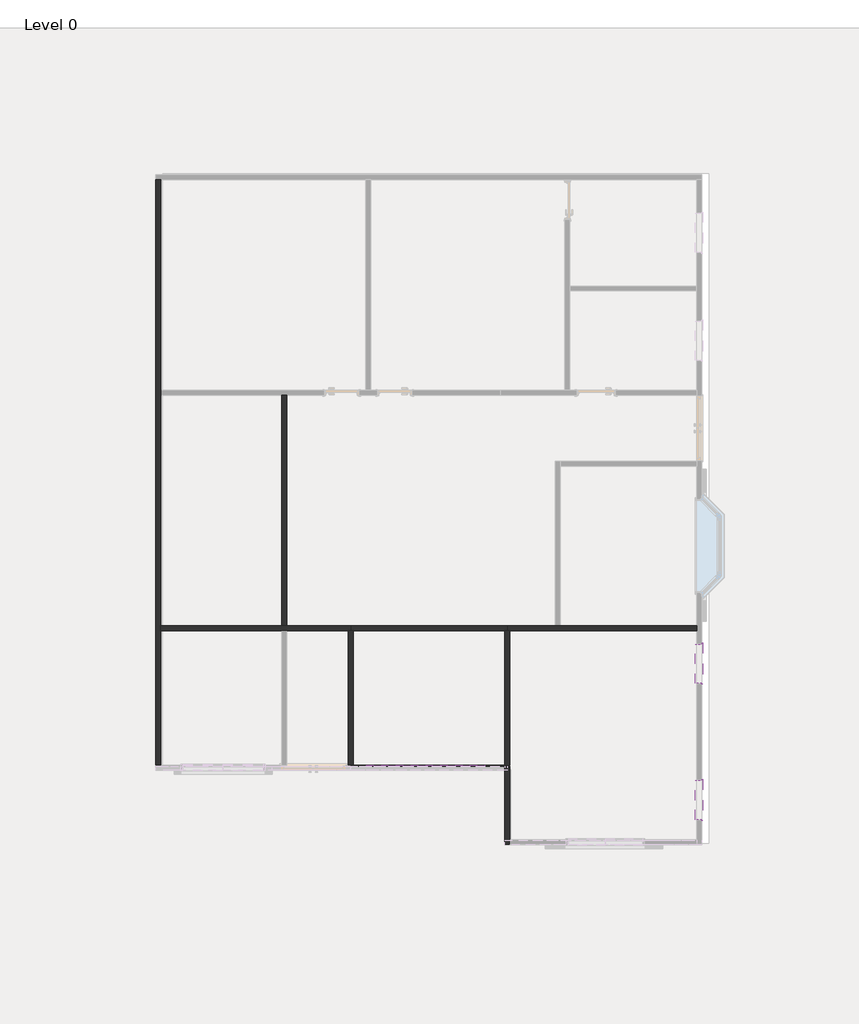
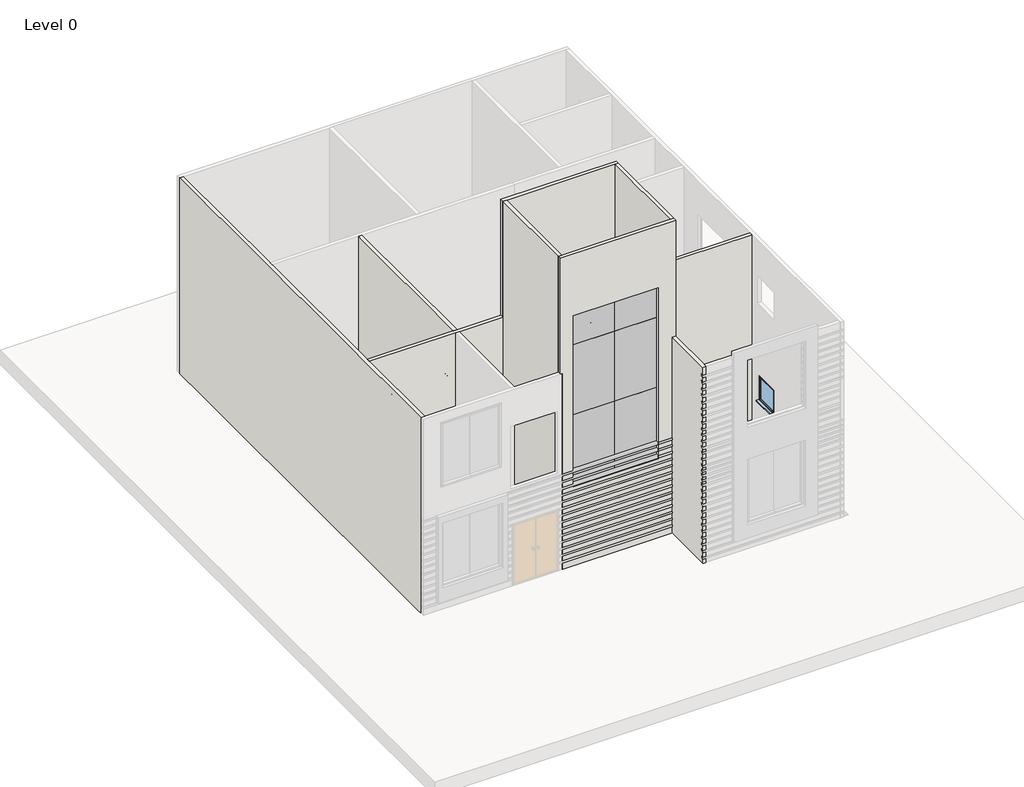
# One storey, part 3 of 5: 10 walls, 6 plates, 2 windows.
"""IFC4 building model written with IfcOpenShell, lengths in millimetres."""

from ifc_helpers import new_model, si_unit, origin, origin_with_axes, place, context, project, spatial, polyline, outline, extrude, faceted_brep, transform, mapped, element, save
from components import system_panel_glazed_fc6345c6, system_panel_glazed_e2854511, windows_sgl_plain_910x910mm_53772929

model = new_model("IFC4")

# Units and contexts
model_context = context("Model", 3, world=origin())
ifc_project = project(units=[si_unit("LENGTHUNIT", "METRE", prefix="MILLI")], contexts=[model_context])

# Site, building, storey
site = spatial("IfcSite", under=ifc_project)
building = spatial("IfcBuilding", under=site)
storey = spatial("IfcBuildingStorey", under=building, Name="Level 0", Elevation=0.0)

# Plates
placement = place(None, origin())
system_panel_glazed_shape = system_panel_glazed_fc6345c6(model_context)
element("IfcPlate", 1, ObjectType="System Panel : Glazed", at=placement, inside=storey, context=model_context, shape_type="MappedRepresentation", body=[
    mapped(system_panel_glazed_shape, transform((-13862.829089, -2815.8968048, 2700.0), x_axis=(1.0, 0.0, 0.0), y_axis=(0.0, 1.0, 0.0), z_axis=(0.0, 0.0, 1.0))),
])
element("IfcPlate", 2, ObjectType="System Panel : Glazed", at=placement, inside=storey, context=model_context, shape_type="MappedRepresentation", body=[
    mapped(system_panel_glazed_shape, transform((-12491.229089, -2815.8968048, 2700.0), x_axis=(1.0, 0.0, 0.0), y_axis=(0.0, 1.0, 0.0), z_axis=(0.0, 0.0, 1.0))),
])
element("IfcPlate", 3, ObjectType="System Panel : Glazed", at=placement, inside=storey, context=model_context, shape_type="MappedRepresentation", body=[
    mapped(system_panel_glazed_shape, transform((-13862.829089, -2815.8968048, 5100.0), x_axis=(1.0, 0.0, 0.0), y_axis=(0.0, 1.0, 0.0), z_axis=(0.0, 0.0, 1.0))),
])
element("IfcPlate", 4, ObjectType="System Panel : Glazed", at=placement, inside=storey, context=model_context, shape_type="MappedRepresentation", body=[
    mapped(system_panel_glazed_shape, transform((-12491.229089, -2815.8968048, 5100.0), x_axis=(1.0, 0.0, 0.0), y_axis=(0.0, 1.0, 0.0), z_axis=(0.0, 0.0, 1.0))),
])
system_panel_glazed_2_shape = system_panel_glazed_e2854511(model_context)
element("IfcPlate", 5, ObjectType="System Panel : Glazed", at=placement, inside=storey, context=model_context, shape_type="MappedRepresentation", body=[
    mapped(system_panel_glazed_2_shape, transform((-13862.829089, -2815.8968048, 7500.0), x_axis=(1.0, 0.0, 0.0), y_axis=(0.0, 1.0, 0.0), z_axis=(0.0, 0.0, 1.0))),
])
element("IfcPlate", 6, ObjectType="System Panel : Glazed", at=placement, inside=storey, context=model_context, shape_type="MappedRepresentation", body=[
    mapped(system_panel_glazed_2_shape, transform((-12491.229089, -2815.8968048, 7500.0), x_axis=(1.0, 0.0, 0.0), y_axis=(0.0, 1.0, 0.0), z_axis=(0.0, 0.0, 1.0))),
])

# Walls
element("IfcWall", 7, ObjectType="basic wall", at=placement, inside=storey, context=model_context, shape_type="Brep", body=[
    faceted_brep([(-19412.729089, 10785.8031952, 0.0), (-19412.729089, -2758.7468048, 0.0), (-19412.729089, -2758.7468048, 6705.6), (-19412.729089, 10785.8031952, 6705.6), (-19298.429089, 10785.8031952, 0.0), (-19298.429089, 10785.8031952, 6705.6), (-19298.429089, 5909.0031952, 6705.6), (-19298.429089, 5794.7031952, 6705.6), (-19298.429089, 460.7031952, 6705.6), (-19298.429089, 346.4031952, 6705.6), (-19298.429089, -2758.7468048, 6705.6), (-19298.429089, -2758.7468048, 0.0), (-19298.429089, 346.4031952, 0.0), (-19298.429089, 460.7031952, 0.0), (-19298.429089, 5794.7031952, 0.0), (-19298.429089, 5909.0031952, 0.0)], [[[0, 1, 2, 3]], [[4, 5, 6, 7, 8, 9, 10, 11, 12, 13, 14, 15]], [[1, 0, 4, 15, 14, 13, 12, 11]], [[3, 2, 10, 9, 8, 7, 6, 5]], [[0, 3, 5, 4]], [[1, 11, 10, 2]]]),
])
element("IfcWall", 8, ObjectType="basic wall", at=placement, inside=storey, context=model_context, shape_type="Brep", body=[
    faceted_brep([(-11348.229089, 346.4031952, 10668.0), (-11348.229089, 346.4031952, 0.0), (-11348.229089, -2758.7468048, 0.0), (-11348.229089, -2758.7468048, 10668.0), (-11233.929089, 346.4031952, 0.0), (-11233.929089, 346.4031952, 6705.6), (-11233.929089, 346.4031952, 10668.0), (-11233.929089, -2758.7468048, 10668.0), (-11233.929089, -2758.7468048, 6705.6), (-11233.929089, -2758.7468048, 0.0), (-11291.079089, 346.4031952, 0.0)], [[[0, 1, 2, 3]], [[4, 5, 6, 7, 8, 9]], [[2, 1, 10, 4, 9]], [[0, 3, 7, 6]], [[0, 6, 5, 4, 10, 1]], [[3, 2, 9, 8, 7]]]),
])
element("IfcWall", 9, ObjectType="basic wall", at=placement, inside=storey, context=model_context, shape_type="Brep", body=[
    faceted_brep([(-6903.229089, 460.7031952, 0.0), (-10065.529089, 460.7031952, 0.0), (-10179.829089, 460.7031952, 0.0), (-11291.079089, 460.7031952, 0.0), (-11291.079089, 460.7031952, 6705.6), (-11233.929089, 460.7031952, 6705.6), (-10179.829089, 460.7031952, 6705.6), (-10065.529089, 460.7031952, 6705.6), (-6903.229089, 460.7031952, 6705.6), (-6903.229089, 346.4031952, 0.0), (-6903.229089, 346.4031952, 6705.6), (-11233.929089, 346.4031952, 6705.6), (-11291.079089, 346.4031952, 6705.6), (-11291.079089, 346.4031952, 0.0), (-11233.929089, 346.4031952, 0.0)], [[[0, 1, 2, 3, 4, 5, 6, 7, 8]], [[9, 10, 11, 12, 13, 14]], [[3, 2, 1, 0, 9, 14, 13]], [[4, 3, 13, 12]], [[8, 7, 6, 5, 4, 12, 11, 10]], [[0, 8, 10, 9]]]),
])
element("IfcWall", 10, ObjectType="basic wall", at=placement, inside=storey, context=model_context, shape_type="Brep", body=[
    faceted_brep([(-14967.729089, 346.4031952, 10668.0), (-14967.729089, 346.4031952, 6705.6), (-14967.729089, 346.4031952, 0.0), (-14967.729089, -2758.7468048, 0.0), (-14967.729089, -2758.7468048, 6705.6), (-14967.729089, -2758.7468048, 10668.0), (-14853.429089, 346.4031952, 0.0), (-14853.429089, 346.4031952, 10668.0), (-14853.429089, -2758.7468048, 10668.0), (-14853.429089, -2758.7468048, 0.0), (-14910.579089, 346.4031952, 0.0), (-14910.579089, -2758.7468048, 0.0)], [[[0, 1, 2, 3, 4, 5]], [[6, 7, 8, 9]], [[3, 2, 10, 6, 9, 11]], [[0, 5, 8, 7]], [[0, 7, 6, 10, 2, 1]], [[3, 11, 9, 8, 5, 4]]]),
])
element("IfcWall", 11, ObjectType="basic wall", at=placement, inside=storey, context=model_context, shape_type="SweptSolid", body=[
    extrude(outline(polyline([(-16504.429089, 460.7031952), (-16504.429089, 5794.7031952), (-16390.129089, 5794.7031952), (-16390.129089, 460.7031952), (-16504.429089, 460.7031952)])), origin_with_axes(), (0.0, 0.0, 1.0), 6705.6),
])
element("IfcWall", 12, ObjectType="basic wall", at=placement, inside=storey, context=model_context, shape_type="Brep", body=[
    faceted_brep([(-14910.579089, 460.7031952, 0.0), (-16390.129089, 460.7031952, 0.0), (-16504.429089, 460.7031952, 0.0), (-19298.429089, 460.7031952, 0.0), (-19298.429089, 460.7031952, 6705.6), (-16504.429089, 460.7031952, 6705.6), (-16390.129089, 460.7031952, 6705.6), (-14967.729089, 460.7031952, 6705.6), (-14910.579089, 460.7031952, 6705.6), (-14910.579089, 346.4031952, 0.0), (-14910.579089, 346.4031952, 6705.6), (-14967.729089, 346.4031952, 6705.6), (-16390.129089, 346.4031952, 6705.6), (-16504.429089, 346.4031952, 6705.6), (-19298.429089, 346.4031952, 6705.6), (-19298.429089, 346.4031952, 0.0), (-16504.429089, 346.4031952, 0.0), (-16390.129089, 346.4031952, 0.0), (-14967.729089, 346.4031952, 0.0)], [[[0, 1, 2, 3, 4, 5, 6, 7, 8]], [[9, 10, 11, 12, 13, 14, 15, 16, 17, 18]], [[3, 2, 1, 0, 9, 18, 17, 16, 15]], [[8, 7, 6, 5, 4, 14, 13, 12, 11, 10]], [[0, 8, 10, 9]], [[4, 3, 15, 14]]]),
])
element("IfcWall", 13, ObjectType="basic wall", at=placement, inside=storey, context=model_context, shape_type="Brep", body=[
    faceted_brep([(-11291.079089, 460.7031952, 0.0), (-14910.579089, 460.7031952, 0.0), (-14910.579089, 460.7031952, 6705.6), (-14967.729089, 460.7031952, 6705.6), (-14967.729089, 460.7031952, 10668.0), (-11233.929089, 460.7031952, 10668.0), (-11233.929089, 460.7031952, 6705.6), (-11291.079089, 460.7031952, 6705.6), (-11291.079089, 346.4031952, 0.0), (-11291.079089, 346.4031952, 6705.6), (-11233.929089, 346.4031952, 6705.6), (-11233.929089, 346.4031952, 10668.0), (-11348.229089, 346.4031952, 10668.0), (-14853.429089, 346.4031952, 10668.0), (-14967.729089, 346.4031952, 10668.0), (-14967.729089, 346.4031952, 6705.6), (-14910.579089, 346.4031952, 6705.6), (-14910.579089, 346.4031952, 0.0), (-14853.429089, 346.4031952, 0.0), (-11348.229089, 346.4031952, 0.0)], [[[0, 1, 2, 3, 4, 5, 6, 7]], [[8, 9, 10, 11, 12, 13, 14, 15, 16, 17, 18, 19]], [[1, 0, 8, 19, 18, 17]], [[5, 4, 14, 13, 12, 11]], [[0, 7, 9, 8]], [[6, 10, 9, 7]], [[6, 5, 11, 10]], [[2, 1, 17, 16]], [[15, 3, 2, 16]], [[4, 3, 15, 14]]]),
])
element("IfcWall", 14, ObjectType="basic wall", at=placement, inside=storey, context=model_context, shape_type="Brep", body=[
    faceted_brep([(-11348.229089, -2815.8968048, 0.0), (-11348.229089, -2873.0468048, 0.0), (-11348.229089, -4593.8968048, 0.0), (-11348.229089, -4593.8968048, 152.4), (-11348.229089, -4501.3968048, 152.4), (-11348.229089, -4501.3968048, 227.4), (-11348.229089, -4583.8968048, 227.4), (-11348.229089, -4593.8968048, 217.4), (-11348.229089, -4593.8968048, 381.0), (-11348.229089, -4501.3968048, 381.0), (-11348.229089, -4501.3968048, 456.0), (-11348.229089, -4583.8968048, 456.0), (-11348.229089, -4593.8968048, 446.0), (-11348.229089, -4593.8968048, 609.6), (-11348.229089, -4501.3968048, 609.6), (-11348.229089, -4501.3968048, 684.6), (-11348.229089, -4583.8968048, 684.6), (-11348.229089, -4593.8968048, 674.6), (-11348.229089, -4593.8968048, 830.4106439), (-11348.229089, -4501.3968048, 830.4106439), (-11348.229089, -4501.3968048, 905.4106439), (-11348.229089, -4583.8968048, 905.4106439), (-11348.229089, -4593.8968048, 895.4106439), (-11348.229089, -4593.8968048, 1059.0106439), (-11348.229089, -4501.3968048, 1059.0106439), (-11348.229089, -4501.3968048, 1134.0106439), (-11348.229089, -4583.8968048, 1134.0106439), (-11348.229089, -4593.8968048, 1124.0106439), (-11348.229089, -4593.8968048, 1279.8212878), (-11348.229089, -4501.3968048, 1279.8212878), (-11348.229089, -4501.3968048, 1354.8212878), (-11348.229089, -4583.8968048, 1354.8212878), (-11348.229089, -4593.8968048, 1344.8212878), (-11348.229089, -4593.8968048, 1500.6319317), (-11348.229089, -4501.3968048, 1500.6319317), (-11348.229089, -4501.3968048, 1575.6319317), (-11348.229089, -4583.8968048, 1575.6319317), (-11348.229089, -4593.8968048, 1565.6319317), (-11348.229089, -4593.8968048, 1729.2319317), (-11348.229089, -4501.3968048, 1729.2319317), (-11348.229089, -4501.3968048, 1804.2319317), (-11348.229089, -4583.8968048, 1804.2319317), (-11348.229089, -4593.8968048, 1794.2319317), (-11348.229089, -4593.8968048, 1957.8319317), (-11348.229089, -4501.3968048, 1957.8319317), (-11348.229089, -4501.3968048, 2032.8319317), (-11348.229089, -4583.8968048, 2032.8319317), (-11348.229089, -4593.8968048, 2022.8319317), (-11348.229089, -4593.8968048, 2186.4319317), (-11348.229089, -4501.3968048, 2186.4319317), (-11348.229089, -4501.3968048, 2261.4319317), (-11348.229089, -4583.8968048, 2261.4319317), (-11348.229089, -4593.8968048, 2251.4319317), (-11348.229089, -4593.8968048, 2415.0319317), (-11348.229089, -4501.3968048, 2415.0319317), (-11348.229089, -4501.3968048, 2490.0319317), (-11348.229089, -4583.8968048, 2490.0319317), (-11348.229089, -4593.8968048, 2480.0319317), (-11348.229089, -4593.8968048, 2643.6319317), (-11348.229089, -4501.3968048, 2643.6319317), (-11348.229089, -4501.3968048, 2718.6319317), (-11348.229089, -4583.8968048, 2718.6319317), (-11348.229089, -4593.8968048, 2708.6319317), (-11348.229089, -4593.8968048, 2805.2765418), (-11348.229089, -4501.3968048, 2805.2765418), (-11348.229089, -4501.3968048, 2880.2765418), (-11348.229089, -4583.8968048, 2880.2765418), (-11348.229089, -4593.8968048, 2870.2765418), (-11348.229089, -4593.8968048, 2966.921152), (-11348.229089, -4501.3968048, 2966.921152), (-11348.229089, -4501.3968048, 3041.921152), (-11348.229089, -4583.8968048, 3041.921152), (-11348.229089, -4593.8968048, 3031.921152), (-11348.229089, -4593.8968048, 3128.5657622), (-11348.229089, -4501.3968048, 3128.5657622), (-11348.229089, -4501.3968048, 3203.5657622), (-11348.229089, -4583.8968048, 3203.5657622), (-11348.229089, -4593.8968048, 3193.5657622), (-11348.229089, -4593.8968048, 3290.2103724), (-11348.229089, -4501.3968048, 3290.2103724), (-11348.229089, -4501.3968048, 3365.2103724), (-11348.229089, -4583.8968048, 3365.2103724), (-11348.229089, -4593.8968048, 3355.2103724), (-11348.229089, -4593.8968048, 3518.8103724), (-11348.229089, -4501.3968048, 3518.8103724), (-11348.229089, -4501.3968048, 3593.8103724), (-11348.229089, -4583.8968048, 3593.8103724), (-11348.229089, -4593.8968048, 3583.8103724), (-11348.229089, -4593.8968048, 3747.4103724), (-11348.229089, -4501.3968048, 3747.4103724), (-11348.229089, -4501.3968048, 3822.4103724), (-11348.229089, -4583.8968048, 3822.4103724), (-11348.229089, -4593.8968048, 3812.4103724), (-11348.229089, -4593.8968048, 3909.0549826), (-11348.229089, -4501.3968048, 3909.0549826), (-11348.229089, -4501.3968048, 3984.0549826), (-11348.229089, -4583.8968048, 3984.0549826), (-11348.229089, -4593.8968048, 3974.0549826), (-11348.229089, -4593.8968048, 4137.6549826), (-11348.229089, -4501.3968048, 4137.6549826), (-11348.229089, -4501.3968048, 4212.6549826), (-11348.229089, -4583.8968048, 4212.6549826), (-11348.229089, -4593.8968048, 4202.6549826), (-11348.229089, -4593.8968048, 4358.4656265), (-11348.229089, -4501.3968048, 4358.4656265), (-11348.229089, -4501.3968048, 4433.4656265), (-11348.229089, -4583.8968048, 4433.4656265), (-11348.229089, -4593.8968048, 4423.4656265), (-11348.229089, -4593.8968048, 4545.5846362), (-11348.229089, -4501.3968048, 4545.5846362), (-11348.229089, -4501.3968048, 4620.5846362), (-11348.229089, -4583.8968048, 4620.5846362), (-11348.229089, -4593.8968048, 4610.5846362), (-11348.229089, -4593.8968048, 4774.1846362), (-11348.229089, -4501.3968048, 4774.1846362), (-11348.229089, -4501.3968048, 4849.1846362), (-11348.229089, -4583.8968048, 4849.1846362), (-11348.229089, -4593.8968048, 4839.1846362), (-11348.229089, -4593.8968048, 5002.7846362), (-11348.229089, -4501.3968048, 5002.7846362), (-11348.229089, -4501.3968048, 5077.7846362), (-11348.229089, -4583.8968048, 5077.7846362), (-11348.229089, -4593.8968048, 5067.7846362), (-11348.229089, -4593.8968048, 5231.3846362), (-11348.229089, -4501.3968048, 5231.3846362), (-11348.229089, -4501.3968048, 5306.3846362), (-11348.229089, -4583.8968048, 5306.3846362), (-11348.229089, -4593.8968048, 5296.3846362), (-11348.229089, -4593.8968048, 5459.9846362), (-11348.229089, -4501.3968048, 5459.9846362), (-11348.229089, -4501.3968048, 5534.9846362), (-11348.229089, -4583.8968048, 5534.9846362), (-11348.229089, -4593.8968048, 5524.9846362), (-11348.229089, -4593.8968048, 5688.5846362), (-11348.229089, -4501.3968048, 5688.5846362), (-11348.229089, -4501.3968048, 5763.5846362), (-11348.229089, -4583.8968048, 5763.5846362), (-11348.229089, -4593.8968048, 5753.5846362), (-11348.229089, -4593.8968048, 5917.1846362), (-11348.229089, -4501.3968048, 5917.1846362), (-11348.229089, -4501.3968048, 5992.1846362), (-11348.229089, -4583.8968048, 5992.1846362), (-11348.229089, -4593.8968048, 5982.1846362), (-11348.229089, -4593.8968048, 6145.7846362), (-11348.229089, -4501.3968048, 6145.7846362), (-11348.229089, -4501.3968048, 6220.7846362), (-11348.229089, -4583.8968048, 6220.7846362), (-11348.229089, -4593.8968048, 6210.7846362), (-11348.229089, -4593.8968048, 6374.3846362), (-11348.229089, -4501.3968048, 6374.3846362), (-11348.229089, -4501.3968048, 6449.3846362), (-11348.229089, -4583.8968048, 6449.3846362), (-11348.229089, -4593.8968048, 6439.3846362), (-11348.229089, -4593.8968048, 6705.6), (-11348.229089, -2873.0468048, 6705.6), (-11348.229089, -2815.8968048, 6705.6), (-11348.229089, -2815.8968048, 3275.4), (-11348.229089, -2815.8968048, 3200.4), (-11348.229089, -2815.8968048, 3046.8), (-11348.229089, -2815.8968048, 2971.8), (-11348.229089, -2815.8968048, 2818.2), (-11348.229089, -2815.8968048, 2743.2), (-11233.929089, -4593.8968048, 0.0), (-11233.929089, -4479.5968048, 0.0), (-11233.929089, -2815.8968048, 0.0), (-11233.929089, -2815.8968048, 6705.6), (-11233.929089, -2873.0468048, 6705.6), (-11233.929089, -4479.5968048, 6705.6), (-11233.929089, -4593.8968048, 6705.6), (-11233.929089, -4593.8968048, 6439.3846362), (-11233.929089, -4583.8968048, 6449.3846362), (-11233.929089, -4501.3968048, 6449.3846362), (-11233.929089, -4501.3968048, 6374.3846362), (-11233.929089, -4593.8968048, 6374.3846362), (-11233.929089, -4593.8968048, 6210.7846362), (-11233.929089, -4583.8968048, 6220.7846362), (-11233.929089, -4501.3968048, 6220.7846362), (-11233.929089, -4501.3968048, 6145.7846362), (-11233.929089, -4593.8968048, 6145.7846362), (-11233.929089, -4593.8968048, 5982.1846362), (-11233.929089, -4583.8968048, 5992.1846362), (-11233.929089, -4501.3968048, 5992.1846362), (-11233.929089, -4501.3968048, 5917.1846362), (-11233.929089, -4593.8968048, 5917.1846362), (-11233.929089, -4593.8968048, 5753.5846362), (-11233.929089, -4583.8968048, 5763.5846362), (-11233.929089, -4501.3968048, 5763.5846362), (-11233.929089, -4501.3968048, 5688.5846362), (-11233.929089, -4593.8968048, 5688.5846362), (-11233.929089, -4593.8968048, 5524.9846362), (-11233.929089, -4583.8968048, 5534.9846362), (-11233.929089, -4501.3968048, 5534.9846362), (-11233.929089, -4501.3968048, 5459.9846362), (-11233.929089, -4593.8968048, 5459.9846362), (-11233.929089, -4593.8968048, 5296.3846362), (-11233.929089, -4583.8968048, 5306.3846362), (-11233.929089, -4501.3968048, 5306.3846362), (-11233.929089, -4501.3968048, 5231.3846362), (-11233.929089, -4593.8968048, 5231.3846362), (-11233.929089, -4593.8968048, 5067.7846362), (-11233.929089, -4583.8968048, 5077.7846362), (-11233.929089, -4501.3968048, 5077.7846362), (-11233.929089, -4501.3968048, 5002.7846362), (-11233.929089, -4593.8968048, 5002.7846362), (-11233.929089, -4593.8968048, 4839.1846362), (-11233.929089, -4583.8968048, 4849.1846362), (-11233.929089, -4501.3968048, 4849.1846362), (-11233.929089, -4501.3968048, 4774.1846362), (-11233.929089, -4593.8968048, 4774.1846362), (-11233.929089, -4593.8968048, 4610.5846362), (-11233.929089, -4583.8968048, 4620.5846362), (-11233.929089, -4501.3968048, 4620.5846362), (-11233.929089, -4501.3968048, 4545.5846362), (-11233.929089, -4593.8968048, 4545.5846362), (-11233.929089, -4593.8968048, 4423.4656265), (-11233.929089, -4583.8968048, 4433.4656265), (-11233.929089, -4501.3968048, 4433.4656265), (-11233.929089, -4501.3968048, 4358.4656265), (-11233.929089, -4593.8968048, 4358.4656265), (-11233.929089, -4593.8968048, 4202.6549826), (-11233.929089, -4583.8968048, 4212.6549826), (-11233.929089, -4501.3968048, 4212.6549826), (-11233.929089, -4501.3968048, 4137.6549826), (-11233.929089, -4593.8968048, 4137.6549826), (-11233.929089, -4593.8968048, 3974.0549826), (-11233.929089, -4583.8968048, 3984.0549826), (-11233.929089, -4501.3968048, 3984.0549826), (-11233.929089, -4501.3968048, 3909.0549826), (-11233.929089, -4593.8968048, 3909.0549826), (-11233.929089, -4593.8968048, 3812.4103724), (-11233.929089, -4583.8968048, 3822.4103724), (-11233.929089, -4501.3968048, 3822.4103724), (-11233.929089, -4501.3968048, 3747.4103724), (-11233.929089, -4593.8968048, 3747.4103724), (-11233.929089, -4593.8968048, 3583.8103724), (-11233.929089, -4583.8968048, 3593.8103724), (-11233.929089, -4501.3968048, 3593.8103724), (-11233.929089, -4501.3968048, 3518.8103724), (-11233.929089, -4593.8968048, 3518.8103724), (-11233.929089, -4593.8968048, 3355.2103724), (-11233.929089, -4583.8968048, 3365.2103724), (-11233.929089, -4501.3968048, 3365.2103724), (-11233.929089, -4501.3968048, 3290.2103724), (-11233.929089, -4593.8968048, 3290.2103724), (-11233.929089, -4593.8968048, 3193.5657622), (-11233.929089, -4583.8968048, 3203.5657622), (-11233.929089, -4501.3968048, 3203.5657622), (-11233.929089, -4501.3968048, 3128.5657622), (-11233.929089, -4593.8968048, 3128.5657622), (-11233.929089, -4593.8968048, 3031.921152), (-11233.929089, -4583.8968048, 3041.921152), (-11233.929089, -4501.3968048, 3041.921152), (-11233.929089, -4501.3968048, 2966.921152), (-11233.929089, -4593.8968048, 2966.921152), (-11233.929089, -4593.8968048, 2870.2765418), (-11233.929089, -4583.8968048, 2880.2765418), (-11233.929089, -4501.3968048, 2880.2765418), (-11233.929089, -4501.3968048, 2805.2765418), (-11233.929089, -4593.8968048, 2805.2765418), (-11233.929089, -4593.8968048, 2708.6319317), (-11233.929089, -4583.8968048, 2718.6319317), (-11233.929089, -4501.3968048, 2718.6319317), (-11233.929089, -4501.3968048, 2643.6319317), (-11233.929089, -4593.8968048, 2643.6319317), (-11233.929089, -4593.8968048, 2480.0319317), (-11233.929089, -4583.8968048, 2490.0319317), (-11233.929089, -4501.3968048, 2490.0319317), (-11233.929089, -4501.3968048, 2415.0319317), (-11233.929089, -4593.8968048, 2415.0319317), (-11233.929089, -4593.8968048, 2251.4319317), (-11233.929089, -4583.8968048, 2261.4319317), (-11233.929089, -4501.3968048, 2261.4319317), (-11233.929089, -4501.3968048, 2186.4319317), (-11233.929089, -4593.8968048, 2186.4319317), (-11233.929089, -4593.8968048, 2022.8319317), (-11233.929089, -4583.8968048, 2032.8319317), (-11233.929089, -4501.3968048, 2032.8319317), (-11233.929089, -4501.3968048, 1957.8319317), (-11233.929089, -4593.8968048, 1957.8319317), (-11233.929089, -4593.8968048, 1794.2319317), (-11233.929089, -4583.8968048, 1804.2319317), (-11233.929089, -4501.3968048, 1804.2319317), (-11233.929089, -4501.3968048, 1729.2319317), (-11233.929089, -4593.8968048, 1729.2319317), (-11233.929089, -4593.8968048, 1565.6319317), (-11233.929089, -4583.8968048, 1575.6319317), (-11233.929089, -4501.3968048, 1575.6319317), (-11233.929089, -4501.3968048, 1500.6319317), (-11233.929089, -4593.8968048, 1500.6319317), (-11233.929089, -4593.8968048, 1344.8212878), (-11233.929089, -4583.8968048, 1354.8212878), (-11233.929089, -4501.3968048, 1354.8212878), (-11233.929089, -4501.3968048, 1279.8212878), (-11233.929089, -4593.8968048, 1279.8212878), (-11233.929089, -4593.8968048, 1124.0106439), (-11233.929089, -4583.8968048, 1134.0106439), (-11233.929089, -4501.3968048, 1134.0106439), (-11233.929089, -4501.3968048, 1059.0106439), (-11233.929089, -4593.8968048, 1059.0106439), (-11233.929089, -4593.8968048, 895.4106439), (-11233.929089, -4583.8968048, 905.4106439), (-11233.929089, -4501.3968048, 905.4106439), (-11233.929089, -4501.3968048, 830.4106439), (-11233.929089, -4593.8968048, 830.4106439), (-11233.929089, -4593.8968048, 674.6), (-11233.929089, -4583.8968048, 684.6), (-11233.929089, -4501.3968048, 684.6), (-11233.929089, -4501.3968048, 609.6), (-11233.929089, -4593.8968048, 609.6), (-11233.929089, -4593.8968048, 446.0), (-11233.929089, -4583.8968048, 456.0), (-11233.929089, -4501.3968048, 456.0), (-11233.929089, -4501.3968048, 381.0), (-11233.929089, -4593.8968048, 381.0), (-11233.929089, -4593.8968048, 217.4), (-11233.929089, -4583.8968048, 227.4), (-11233.929089, -4501.3968048, 227.4), (-11233.929089, -4501.3968048, 152.4), (-11233.929089, -4593.8968048, 152.4)], [[[0, 1, 2, 3, 4, 5, 6, 7, 8, 9, 10, 11, 12, 13, 14, 15, 16, 17, 18, 19, 20, 21, 22, 23, 24, 25, 26, 27, 28, 29, 30, 31, 32, 33, 34, 35, 36, 37, 38, 39, 40, 41, 42, 43, 44, 45, 46, 47, 48, 49, 50, 51, 52, 53, 54, 55, 56, 57, 58, 59, 60, 61, 62, 63, 64, 65, 66, 67, 68, 69, 70, 71, 72, 73, 74, 75, 76, 77, 78, 79, 80, 81, 82, 83, 84, 85, 86, 87, 88, 89, 90, 91, 92, 93, 94, 95, 96, 97, 98, 99, 100, 101, 102, 103, 104, 105, 106, 107, 108, 109, 110, 111, 112, 113, 114, 115, 116, 117, 118, 119, 120, 121, 122, 123, 124, 125, 126, 127, 128, 129, 130, 131, 132, 133, 134, 135, 136, 137, 138, 139, 140, 141, 142, 143, 144, 145, 146, 147, 148, 149, 150, 151, 152, 153, 154, 155, 156, 157, 158, 159, 160, 161]], [[162, 163, 164, 165, 166, 167, 168, 169, 170, 171, 172, 173, 174, 175, 176, 177, 178, 179, 180, 181, 182, 183, 184, 185, 186, 187, 188, 189, 190, 191, 192, 193, 194, 195, 196, 197, 198, 199, 200, 201, 202, 203, 204, 205, 206, 207, 208, 209, 210, 211, 212, 213, 214, 215, 216, 217, 218, 219, 220, 221, 222, 223, 224, 225, 226, 227, 228, 229, 230, 231, 232, 233, 234, 235, 236, 237, 238, 239, 240, 241, 242, 243, 244, 245, 246, 247, 248, 249, 250, 251, 252, 253, 254, 255, 256, 257, 258, 259, 260, 261, 262, 263, 264, 265, 266, 267, 268, 269, 270, 271, 272, 273, 274, 275, 276, 277, 278, 279, 280, 281, 282, 283, 284, 285, 286, 287, 288, 289, 290, 291, 292, 293, 294, 295, 296, 297, 298, 299, 300, 301, 302, 303, 304, 305, 306, 307, 308, 309, 310, 311, 312, 313, 314, 315, 316, 317, 318]], [[2, 1, 0, 164, 163, 162]], [[155, 154, 153, 168, 167, 166, 165]], [[165, 164, 0, 161, 160, 159, 158, 157, 156, 155]], [[2, 162, 318, 3]], [[168, 153, 152, 169]], [[7, 314, 313, 8]], [[12, 309, 308, 13]], [[17, 304, 303, 18]], [[22, 299, 298, 23]], [[27, 294, 293, 28]], [[32, 289, 288, 33]], [[37, 284, 283, 38]], [[42, 279, 278, 43]], [[47, 274, 273, 48]], [[52, 269, 268, 53]], [[57, 264, 263, 58]], [[62, 259, 258, 63]], [[67, 254, 253, 68]], [[72, 249, 248, 73]], [[77, 244, 243, 78]], [[82, 239, 238, 83]], [[87, 234, 233, 88]], [[92, 229, 228, 93]], [[97, 224, 223, 98]], [[102, 219, 218, 103]], [[107, 214, 213, 108]], [[112, 209, 208, 113]], [[117, 204, 203, 118]], [[122, 199, 198, 123]], [[127, 194, 193, 128]], [[132, 189, 188, 133]], [[137, 184, 183, 138]], [[142, 179, 178, 143]], [[147, 174, 173, 148]], [[317, 4, 3, 318]], [[6, 315, 314, 7]], [[315, 6, 5, 316]], [[4, 317, 316, 5]], [[312, 9, 8, 313]], [[11, 310, 309, 12]], [[310, 11, 10, 311]], [[9, 312, 311, 10]], [[307, 14, 13, 308]], [[16, 305, 304, 17]], [[305, 16, 15, 306]], [[14, 307, 306, 15]], [[302, 19, 18, 303]], [[21, 300, 299, 22]], [[300, 21, 20, 301]], [[19, 302, 301, 20]], [[297, 24, 23, 298]], [[26, 295, 294, 27]], [[295, 26, 25, 296]], [[24, 297, 296, 25]], [[292, 29, 28, 293]], [[31, 290, 289, 32]], [[290, 31, 30, 291]], [[29, 292, 291, 30]], [[287, 34, 33, 288]], [[36, 285, 284, 37]], [[285, 36, 35, 286]], [[34, 287, 286, 35]], [[282, 39, 38, 283]], [[41, 280, 279, 42]], [[280, 41, 40, 281]], [[39, 282, 281, 40]], [[277, 44, 43, 278]], [[46, 275, 274, 47]], [[275, 46, 45, 276]], [[44, 277, 276, 45]], [[272, 49, 48, 273]], [[51, 270, 269, 52]], [[270, 51, 50, 271]], [[49, 272, 271, 50]], [[267, 54, 53, 268]], [[56, 265, 264, 57]], [[265, 56, 55, 266]], [[54, 267, 266, 55]], [[262, 59, 58, 263]], [[61, 260, 259, 62]], [[260, 61, 60, 261]], [[59, 262, 261, 60]], [[257, 64, 63, 258]], [[66, 255, 254, 67]], [[255, 66, 65, 256]], [[64, 257, 256, 65]], [[252, 69, 68, 253]], [[71, 250, 249, 72]], [[250, 71, 70, 251]], [[69, 252, 251, 70]], [[247, 74, 73, 248]], [[76, 245, 244, 77]], [[245, 76, 75, 246]], [[74, 247, 246, 75]], [[242, 79, 78, 243]], [[81, 240, 239, 82]], [[240, 81, 80, 241]], [[79, 242, 241, 80]], [[237, 84, 83, 238]], [[86, 235, 234, 87]], [[235, 86, 85, 236]], [[84, 237, 236, 85]], [[232, 89, 88, 233]], [[91, 230, 229, 92]], [[230, 91, 90, 231]], [[89, 232, 231, 90]], [[227, 94, 93, 228]], [[96, 225, 224, 97]], [[225, 96, 95, 226]], [[94, 227, 226, 95]], [[222, 99, 98, 223]], [[101, 220, 219, 102]], [[220, 101, 100, 221]], [[99, 222, 221, 100]], [[217, 104, 103, 218]], [[106, 215, 214, 107]], [[215, 106, 105, 216]], [[104, 217, 216, 105]], [[212, 109, 108, 213]], [[111, 210, 209, 112]], [[210, 111, 110, 211]], [[109, 212, 211, 110]], [[207, 114, 113, 208]], [[116, 205, 204, 117]], [[205, 116, 115, 206]], [[114, 207, 206, 115]], [[202, 119, 118, 203]], [[121, 200, 199, 122]], [[200, 121, 120, 201]], [[119, 202, 201, 120]], [[197, 124, 123, 198]], [[126, 195, 194, 127]], [[195, 126, 125, 196]], [[124, 197, 196, 125]], [[192, 129, 128, 193]], [[131, 190, 189, 132]], [[190, 131, 130, 191]], [[129, 192, 191, 130]], [[187, 134, 133, 188]], [[136, 185, 184, 137]], [[185, 136, 135, 186]], [[134, 187, 186, 135]], [[182, 139, 138, 183]], [[141, 180, 179, 142]], [[180, 141, 140, 181]], [[139, 182, 181, 140]], [[177, 144, 143, 178]], [[146, 175, 174, 147]], [[175, 146, 145, 176]], [[144, 177, 176, 145]], [[172, 149, 148, 173]], [[151, 170, 169, 152]], [[170, 151, 150, 171]], [[149, 172, 171, 150]]]),
])
element("IfcWall", 15, ObjectType="basic wall", at=placement, inside=storey, context=model_context, shape_type="Brep", body=[
    faceted_brep([(-11348.229089, -2790.4968048, 0.0), (-11348.229089, -2815.8968048, 0.0), (-11348.229089, -2815.8968048, 2743.2), (-11348.229089, -2815.8968048, 2818.2), (-11348.229089, -2815.8968048, 2971.8), (-11348.229089, -2815.8968048, 3046.8), (-11348.229089, -2815.8968048, 3200.4), (-11348.229089, -2815.8968048, 3275.4), (-11348.229089, -2815.8968048, 6705.6), (-11348.229089, -2790.4968048, 6705.6), (-11348.229089, -2790.4968048, 3275.4), (-11348.229089, -2790.4968048, 3200.4), (-11348.229089, -2790.4968048, 3046.8), (-11348.229089, -2790.4968048, 2971.8), (-11348.229089, -2790.4968048, 2818.2), (-11348.229089, -2790.4968048, 2743.2), (-11233.929089, -2790.4968048, 0.0), (-11233.929089, -2790.4968048, 6705.6), (-11233.929089, -2815.8968048, 6705.6), (-11233.929089, -2815.8968048, 0.0)], [[[0, 1, 2, 3, 4, 5, 6, 7, 8, 9, 10, 11, 12, 13, 14, 15]], [[16, 17, 18, 19]], [[1, 0, 16, 19]], [[8, 7, 6, 5, 4, 3, 2, 1, 19, 18]], [[9, 8, 18, 17]], [[0, 15, 14, 13, 12, 11, 10, 9, 17, 16]]]),
])
element("IfcWall", 16, ObjectType="basic wall", at=placement, inside=storey, context=model_context, shape_type="Brep", body=[
    faceted_brep([(-14910.579089, -2873.0468048, 0.0), (-11348.229089, -2873.0468048, 0.0), (-11348.229089, -2873.0468048, 228.6), (-14910.579089, -2873.0468048, 228.6), (-11233.929089, -2873.0468048, 10668.0), (-14967.729089, -2873.0468048, 10668.0), (-14967.729089, -2873.0468048, 6705.6), (-14910.579089, -2873.0468048, 6705.6), (-14910.579089, -2873.0468048, 3265.4), (-14910.579089, -2873.0468048, 3242.6284072), (-14910.579089, -2873.0468048, 3200.4), (-14910.579089, -2873.0468048, 3177.6284072), (-14910.579089, -2873.0468048, 3036.8), (-14910.579089, -2873.0468048, 3014.0284072), (-14910.579089, -2873.0468048, 2971.8), (-14910.579089, -2873.0468048, 2949.0284072), (-14910.579089, -2873.0468048, 2808.2), (-14910.579089, -2873.0468048, 2785.4284072), (-14910.579089, -2873.0468048, 2743.2), (-14910.579089, -2873.0468048, 2720.4284072), (-14910.579089, -2873.0468048, 2579.6), (-11348.229089, -2873.0468048, 2579.6), (-11348.229089, -2873.0468048, 2743.2), (-11348.229089, -2873.0468048, 2808.2), (-11348.229089, -2873.0468048, 2971.8), (-11348.229089, -2873.0468048, 3036.8), (-11348.229089, -2873.0468048, 3200.4), (-11348.229089, -2873.0468048, 3265.4), (-11348.229089, -2873.0468048, 6705.6), (-11233.929089, -2873.0468048, 6705.6), (-14548.629089, -2873.0468048, 8557.5402127), (-11805.429089, -2873.0468048, 8557.5402127), (-11805.429089, -2873.0468048, 3265.4), (-11805.429089, -2873.0468048, 3200.4), (-11805.429089, -2873.0468048, 3036.8), (-11805.429089, -2873.0468048, 2971.8), (-11805.429089, -2873.0468048, 2808.2), (-11805.429089, -2873.0468048, 2743.2), (-11805.429089, -2873.0468048, 2700.0), (-14548.629089, -2873.0468048, 2700.0), (-14548.629089, -2873.0468048, 2743.2), (-14548.629089, -2873.0468048, 2808.2), (-14548.629089, -2873.0468048, 2971.8), (-14548.629089, -2873.0468048, 3036.8), (-14548.629089, -2873.0468048, 3200.4), (-14548.629089, -2873.0468048, 3265.4), (-11348.229089, -2873.0468048, 1828.8), (-14910.579089, -2873.0468048, 1828.8), (-14910.579089, -2873.0468048, 1821.0106439), (-14910.579089, -2873.0468048, 1665.2), (-11348.229089, -2873.0468048, 1665.2), (-14910.579089, -2873.0468048, 1893.8), (-11348.229089, -2873.0468048, 1893.8), (-11348.229089, -2873.0468048, 2057.4), (-14910.579089, -2873.0468048, 2057.4), (-14910.579089, -2873.0468048, 2049.6106439), (-14910.579089, -2873.0468048, 2122.4), (-11348.229089, -2873.0468048, 2122.4), (-11348.229089, -2873.0468048, 2286.0), (-14910.579089, -2873.0468048, 2286.0), (-14910.579089, -2873.0468048, 2278.2106439), (-14910.579089, -2873.0468048, 2351.0), (-11348.229089, -2873.0468048, 2351.0), (-11348.229089, -2873.0468048, 2514.6), (-14910.579089, -2873.0468048, 2514.6), (-14910.579089, -2873.0468048, 2506.8106439), (-11348.229089, -2873.0468048, 1436.6), (-11348.229089, -2873.0468048, 1600.2), (-14910.579089, -2873.0468048, 1600.2), (-14910.579089, -2873.0468048, 1436.6), (-11348.229089, -2873.0468048, 1208.0), (-11348.229089, -2873.0468048, 1371.6), (-14910.579089, -2873.0468048, 1371.6), (-14910.579089, -2873.0468048, 1208.0), (-11348.229089, -2873.0468048, 979.4), (-11348.229089, -2873.0468048, 1143.0), (-14910.579089, -2873.0468048, 1143.0), (-14910.579089, -2873.0468048, 979.4), (-11348.229089, -2873.0468048, 750.8), (-11348.229089, -2873.0468048, 914.4), (-14910.579089, -2873.0468048, 914.4), (-14910.579089, -2873.0468048, 750.8), (-11348.229089, -2873.0468048, 522.2), (-11348.229089, -2873.0468048, 685.8), (-14910.579089, -2873.0468048, 685.8), (-14910.579089, -2873.0468048, 522.2), (-11348.229089, -2873.0468048, 293.6), (-11348.229089, -2873.0468048, 457.2), (-14910.579089, -2873.0468048, 457.2), (-14910.579089, -2873.0468048, 293.6), (-11348.229089, -2758.7468048, 0.0), (-14853.429089, -2758.7468048, 0.0), (-14910.579089, -2758.7468048, 0.0), (-14910.579089, -2758.7468048, 6705.6), (-14967.729089, -2758.7468048, 6705.6), (-14967.729089, -2758.7468048, 10668.0), (-14853.429089, -2758.7468048, 10668.0), (-11348.229089, -2758.7468048, 10668.0), (-11233.929089, -2758.7468048, 10668.0), (-11233.929089, -2758.7468048, 6705.6), (-11348.229089, -2758.7468048, 6705.6), (-14548.629089, -2758.7468048, 8557.5402127), (-14548.629089, -2758.7468048, 2700.0), (-11805.429089, -2758.7468048, 2700.0), (-11805.429089, -2758.7468048, 8557.5402127), (-11348.229089, -2790.4968048, 0.0), (-11348.229089, -2815.8968048, 0.0), (-14910.579089, -2780.5468048, 228.6), (-14910.579089, -2780.5468048, 303.6), (-14910.579089, -2863.0468048, 303.6), (-14910.579089, -2780.5468048, 457.2), (-14910.579089, -2780.5468048, 532.2), (-14910.579089, -2863.0468048, 532.2), (-14910.579089, -2780.5468048, 685.8), (-14910.579089, -2780.5468048, 760.8), (-14910.579089, -2863.0468048, 760.8), (-14910.579089, -2780.5468048, 914.4), (-14910.579089, -2780.5468048, 989.4), (-14910.579089, -2863.0468048, 989.4), (-14910.579089, -2780.5468048, 1143.0), (-14910.579089, -2780.5468048, 1218.0), (-14910.579089, -2863.0468048, 1218.0), (-14910.579089, -2780.5468048, 1371.6), (-14910.579089, -2780.5468048, 1446.6), (-14910.579089, -2863.0468048, 1446.6), (-14910.579089, -2780.5468048, 1600.2), (-14910.579089, -2780.5468048, 1675.2), (-14910.579089, -2863.0468048, 1675.2), (-14910.579089, -2780.5468048, 1828.8), (-14910.579089, -2780.5468048, 1896.0106439), (-14910.579089, -2780.5468048, 1903.8), (-14910.579089, -2863.0468048, 1903.8), (-14910.579089, -2780.5468048, 2057.4), (-14910.579089, -2780.5468048, 2124.6106439), (-14910.579089, -2780.5468048, 2132.4), (-14910.579089, -2863.0468048, 2132.4), (-14910.579089, -2780.5468048, 2286.0), (-14910.579089, -2780.5468048, 2353.2106439), (-14910.579089, -2780.5468048, 2361.0), (-14910.579089, -2863.0468048, 2361.0), (-14910.579089, -2780.5468048, 2514.6), (-14910.579089, -2780.5468048, 2581.8106439), (-14910.579089, -2780.5468048, 2589.6), (-14910.579089, -2863.0468048, 2589.6), (-11348.229089, -2815.8968048, 6705.6), (-11348.229089, -2790.4968048, 6705.6), (-11233.929089, -2790.4968048, 6705.6), (-11233.929089, -2815.8968048, 6705.6), (-11348.229089, -2863.0468048, 2589.6), (-11348.229089, -2780.5468048, 2589.6), (-11348.229089, -2780.5468048, 2514.6), (-11348.229089, -2863.0468048, 2361.0), (-11348.229089, -2780.5468048, 2361.0), (-11348.229089, -2780.5468048, 2286.0), (-11348.229089, -2863.0468048, 2132.4), (-11348.229089, -2780.5468048, 2132.4), (-11348.229089, -2780.5468048, 2057.4), (-11348.229089, -2863.0468048, 1903.8), (-11348.229089, -2780.5468048, 1903.8), (-11348.229089, -2780.5468048, 1828.8), (-11348.229089, -2863.0468048, 1675.2), (-11348.229089, -2780.5468048, 1675.2), (-11348.229089, -2780.5468048, 1600.2), (-11348.229089, -2863.0468048, 1446.6), (-11348.229089, -2780.5468048, 1446.6), (-11348.229089, -2780.5468048, 1371.6), (-11348.229089, -2863.0468048, 1218.0), (-11348.229089, -2780.5468048, 1218.0), (-11348.229089, -2780.5468048, 1143.0), (-11348.229089, -2863.0468048, 989.4), (-11348.229089, -2780.5468048, 989.4), (-11348.229089, -2780.5468048, 914.4), (-11348.229089, -2863.0468048, 760.8), (-11348.229089, -2780.5468048, 760.8), (-11348.229089, -2780.5468048, 685.8), (-11348.229089, -2863.0468048, 532.2), (-11348.229089, -2780.5468048, 532.2), (-11348.229089, -2780.5468048, 457.2), (-11348.229089, -2863.0468048, 303.6), (-11348.229089, -2780.5468048, 303.6), (-11348.229089, -2780.5468048, 228.6)], [[[0, 1, 2, 3]], [[4, 5, 6, 7, 8, 9, 10, 11, 12, 13, 14, 15, 16, 17, 18, 19, 20, 21, 22, 23, 24, 25, 26, 27, 28, 29], [30, 31, 32, 33, 34, 35, 36, 37, 38, 39, 40, 41, 42, 43, 44, 45]], [[46, 47, 48, 49, 50]], [[51, 52, 53, 54, 55]], [[56, 57, 58, 59, 60]], [[61, 62, 63, 64, 65]], [[66, 67, 68, 69]], [[70, 71, 72, 73]], [[74, 75, 76, 77]], [[78, 79, 80, 81]], [[82, 83, 84, 85]], [[86, 87, 88, 89]], [[90, 91, 92, 93, 94, 95, 96, 97, 98, 99, 100], [101, 102, 103, 104]], [[1, 0, 92, 91, 90, 105, 106]], [[5, 4, 98, 97, 96, 95]], [[92, 0, 3, 107, 108, 109, 89, 88, 110, 111, 112, 85, 84, 113, 114, 115, 81, 80, 116, 117, 118, 77, 76, 119, 120, 121, 73, 72, 122, 123, 124, 69, 68, 125, 126, 127, 49, 48, 47, 128, 129, 130, 131, 51, 55, 54, 132, 133, 134, 135, 56, 60, 59, 136, 137, 138, 139, 61, 65, 64, 140, 141, 142, 143, 20, 19, 18, 17, 16, 15, 14, 13, 12, 11, 10, 9, 8, 7, 93]], [[94, 93, 7, 6]], [[6, 5, 95, 94]], [[29, 28, 144, 145, 100, 99, 146, 147]], [[1, 106, 105, 90, 100, 145, 144, 28, 27, 26, 25, 24, 23, 22, 21, 148, 149, 150, 63, 62, 151, 152, 153, 58, 57, 154, 155, 156, 53, 52, 157, 158, 159, 46, 50, 160, 161, 162, 67, 66, 163, 164, 165, 71, 70, 166, 167, 168, 75, 74, 169, 170, 171, 79, 78, 172, 173, 174, 83, 82, 175, 176, 177, 87, 86, 178, 179, 180, 2]], [[98, 4, 29, 147, 146, 99]], [[39, 102, 101, 30, 45, 44, 43, 42, 41, 40]], [[30, 101, 104, 31]], [[103, 38, 37, 36, 35, 34, 33, 32, 31, 104]], [[102, 39, 38, 103]], [[128, 159, 158, 130, 129]], [[159, 128, 47, 46]], [[131, 157, 52, 51]], [[157, 131, 130, 158]], [[156, 132, 54, 53]], [[135, 154, 57, 56]], [[154, 135, 134, 155]], [[132, 156, 155, 134, 133]], [[59, 58, 153, 136]], [[62, 61, 139, 151]], [[139, 138, 152, 151]], [[153, 152, 138, 137, 136]], [[64, 63, 150, 140]], [[21, 20, 143, 148]], [[143, 142, 149, 148]], [[150, 149, 142, 141, 140]], [[162, 125, 68, 67]], [[127, 160, 50, 49]], [[160, 127, 126, 161]], [[125, 162, 161, 126]], [[165, 122, 72, 71]], [[124, 163, 66, 69]], [[163, 124, 123, 164]], [[122, 165, 164, 123]], [[168, 119, 76, 75]], [[121, 166, 70, 73]], [[166, 121, 120, 167]], [[119, 168, 167, 120]], [[171, 116, 80, 79]], [[118, 169, 74, 77]], [[169, 118, 117, 170]], [[116, 171, 170, 117]], [[174, 113, 84, 83]], [[115, 172, 78, 81]], [[172, 115, 114, 173]], [[113, 174, 173, 114]], [[177, 110, 88, 87]], [[112, 175, 82, 85]], [[175, 112, 111, 176]], [[110, 177, 176, 111]], [[180, 107, 3, 2]], [[109, 178, 86, 89]], [[178, 109, 108, 179]], [[107, 180, 179, 108]]]),
])

# Windows
windows_sgl_plain_910x910mm_shape = windows_sgl_plain_910x910mm_53772929(model_context)
element("IfcWindow", 17, ObjectType="Windows_Sgl_Plain : 910x910mm", at=placement, inside=storey, context=model_context, shape_type="MappedRepresentation", body=[
    mapped(windows_sgl_plain_910x910mm_shape, transform((-6837.6225212, -413.3968048, 0.0), x_axis=(0.0, 1.0, 0.0), y_axis=(-1.0, 0.0, 0.0), z_axis=(0.0, 0.0, 1.0))),
])
element("IfcWindow", 18, ObjectType="Windows_Sgl_Plain : 910x910mm", at=placement, inside=storey, context=model_context, shape_type="MappedRepresentation", body=[
    mapped(windows_sgl_plain_910x910mm_shape, transform((-6837.6225212, -3567.3968048, 0.0), x_axis=(0.0, 1.0, 0.0), y_axis=(-1.0, 0.0, 0.0), z_axis=(0.0, 0.0, 1.0))),
])

save(model, "model.ifc")

# Revit data of these elements
# Type "System Panel : Glazed"
#   Keynote = "H11"
#   Construction Type Id = "GSP4R"
#   Analytic Construction = "1/8 in Pilkington single glazing"
#   Visual Light Transmittance = 0.9
#   Solar Heat Gain Coefficient = 0.86
#   Heat Transfer Coefficient (U) = 6.7069 W/(m²·K)
#   Define Thermal Properties by = 1
# Type "basic wall"
#   Keynote = "F10"
#   Layers, outside or top first: 0' - 4 1/2" "Air" (function 1)
# Type "Windows_Sgl_Plain : 910x910mm"
#   Type Mark = "44"
#   Operation = "SinglePanel"
#   Construction Type Id = "SGL"
#   Manufacturer = "Revit"
#   Keynote = "L10"
#   Analytic Construction = "Large single-glazed windows"
#   Wrap Layers (Ext) from Ext = 0' - 4.03543"
#   Wrap Layers (Int) from Ext = 0' - 6.98819"
#   Window Board Projection = 0' - 0.98425"
#   Window Board Extension = 0' - 0.98425"
#   Visual Light Transmittance = 0.9
#   Solar Heat Gain Coefficient = 0.86
#   Rough Width = 2' - 11.82677"
#   Rough Height = 2' - 11.82677"
#   Height = 2' - 11.82677"
#   Width = 2' - 11.82677"
#   Heat Transfer Coefficient (U) = 5.5617 W/(m²·K)
#   Glazing Thickness = 0' - 0.94488"
#   FrameOffset - External = 0' - 1.9685"
#   Frame Depth = 0' - 2.55906"
#   Default Head Height = 6' - 11.07087"
#   Cill Depth = 0' - 3.44488"
#   Cavity Closer Width = 0' - 1.9685"
#   Cavity Closer Offset from Ext = 0' - 4.03543"
#   Cavity Closer Depth = 0' - 3.34646"
#   Define Thermal Properties by = 1
#   Vis - Cavity Closers = yes
#   Define Thermal Properties by = 1
#   Material Trim = Window Frame
#   Material Glass = Glass
#   Material Frame = Window Frame
#   Wall Closure = (empty or 0)
# Elements 1, 2, 3, 4, 5, 6 (IfcPlate, "System Panel : Glazed")
#   Phase Created = New Construction
#   Materials on its faces: "Glass"
# Elements 7, 9, 11, 12, 14, 15 (IfcWall, "basic wall")
#   Top Offset = 0' - 0"
#   Base Offset = 0' - 0"
#   wall height = 22' - 0"
#   Phase Created = New Construction
#   Base Constraint = Level 0
#   Top Constraint = Level 2
#   Materials on its faces: "Air"
# Elements 8, 10, 13, 16 (IfcWall, "basic wall")
#   Top Offset = 2' - 0"
#   Base Offset = 0' - 0"
#   wall height = 35' - 0"
#   Phase Created = New Construction
#   Base Constraint = Level 0
#   Top Constraint = Level 3
#   Materials on its faces: "Air"
# Element 17 (IfcWindow, "Windows_Sgl_Plain : 910x910mm")
#   Mark = "2"
#   Phase Created = New Construction
#   Materials on its faces: "Window Frame", "Glass"
# Element 18 (IfcWindow, "Windows_Sgl_Plain : 910x910mm")
#   Mark = "3"
#   Phase Created = New Construction
#   Materials on its faces: "Window Frame", "Glass"
# Materials
#   "Air": class "Gas", colour RGB 255 255 255, transparency 0, Description = "Air", Cost = 0
#   "Window Frame": colour RGB 249 249 249, transparency 0, Keynote = "L10", Cost = 0
#   "Glass": class "Glass", colour RGB 0 128 192, transparency 0.9, Description = "Soda Lime Glass", Cost = 0
